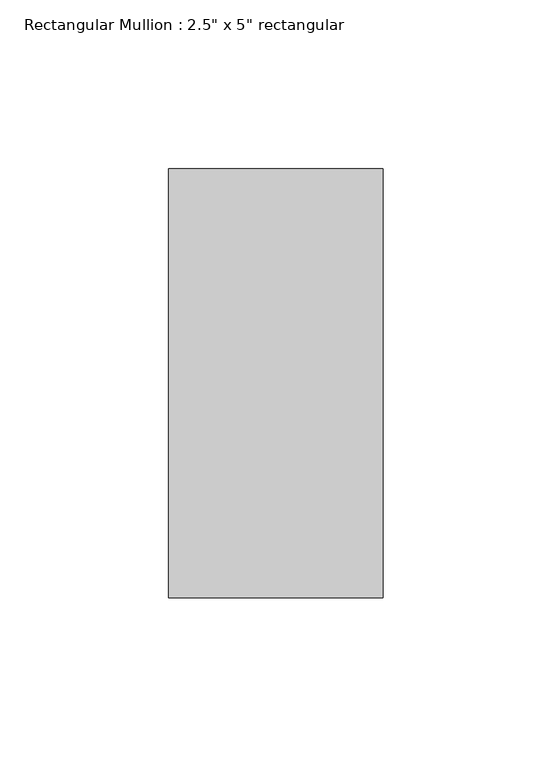
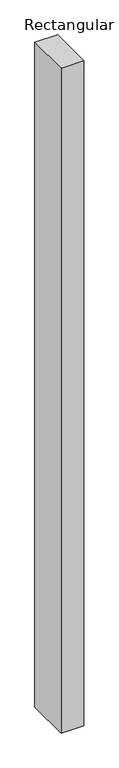
"""IFC4 building model written with IfcOpenShell, lengths in millimetres: member geometry."""

from ifc_helpers import new_model, si_unit, frame, origin, place, context, project, spatial, polyline, outline, extrude, source, transform, mapped, element, save


def member_37619358(model_context):
    return source(origin(), model_context, "Body", "SweptSolid", [
        extrude(outline(polyline([(0.0, 63.5), (0.0, -63.5), (-63.5, -63.5), (-63.5, 63.5), (0.0, 63.5)])), frame((0.0, 0.0, -1970.7905078), z_axis=(0.0, 0.0, 1.0), x_axis=(1.0, 0.0, 0.0)), (0.0, 0.0, 1.0), 1970.7905078),
    ])


if __name__ == "__main__":
    model = new_model("IFC4")
    model_context = context("Model", 3, world=origin())
    ifc_project = project(units=[si_unit("LENGTHUNIT", "METRE", prefix="MILLI")], contexts=[model_context])
    site = spatial("IfcSite", under=ifc_project)
    building = spatial("IfcBuilding", under=site)
    placement = place(None, origin())
    member_shape = member_37619358(model_context)
    element("IfcMember", 1, ObjectType="Rectangular Mullion : 2.5\" x 5\" rectangular", at=placement, inside=building, context=model_context, shape_type="MappedRepresentation", body=[
        mapped(member_shape, transform((0.0, 0.0, 0.0), x_axis=(1.0, 0.0, 0.0), y_axis=(0.0, 1.0, 0.0), z_axis=(0.0, 0.0, 1.0))),
    ])
    save(model, "model.ifc")

# Revit data of these elements
# Type "Rectangular Mullion : 2.5\" x 5\" rectangular"
#   built-in parameter 1007304 = 0.416667 (stored number, unit not read)
#   built-in parameter 1007301 = 0.104167 (stored number, unit not read)
#   built-in parameter 1007300 = 0.104167 (stored number, unit not read)
# Element 1 (IfcMember, "Rectangular Mullion : 2.5\" x 5\" rectangular")
#   Materials on its faces: "Aluminum"
# Materials
#   "Aluminum": class "Metal", colour RGB 247 247 247, transparency 0, Description = "Aluminum 6061", Cost = 0
